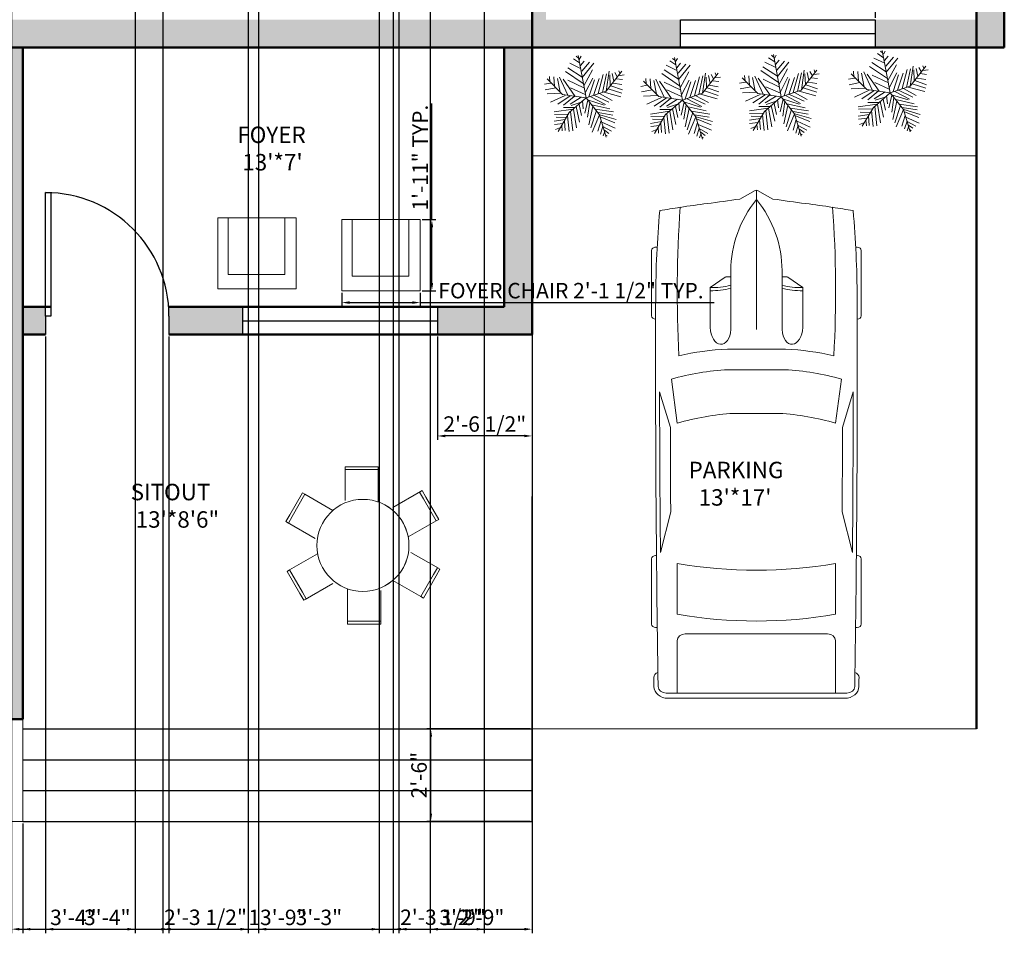
# Model space of a CAD drawing. Units: inches. Extents: x 2152 to 2718, y 1095 to 1798.
# Tile 2 of 5: x 2356 to 2675, y 1095 to 1394. Entities that reach past the tile are written whole.
import ezdxf

# ---------------------------------------------------------------- set-up
doc = ezdxf.new("R2010")
doc.units = ezdxf.units.IN
for name, color, linetype, lineweight in [('A-ANNO-DIMS', 130, 'Continuous', 18), ('A-AREA-IDEN', 130, 'Continuous', 25), ('A-FLOR-STRS', 7, 'Continuous', 25), ('A-WALL-PATT', 210, 'Continuous', 13), ('C-PRKG-VEHI', 8, 'Continuous', 13), ('DOOR', 160, 'Continuous', 25), ('FUR', 10, 'Continuous', 18), ('L-HRDS', 8, 'Continuous', 20), ('L-PLNT-BEDS', 80, 'Continuous', 18), ('TREE', 80, 'Continuous', 13), ('WALL', 7, 'Continuous', 50), ('WIND', 140, 'Continuous', 25)]:
    doc.layers.add(name, color=color, linetype=linetype, lineweight=lineweight)
doc.styles.get("Standard").update_dxf_attribs({"font": 'arial.ttf'})
doc.dimstyles.new('ISO-25', dxfattribs={"dimtxt": 5, "dimasz": 2.5, "dimexe": 1.25, "dimexo": 0.625, "dimtad": 1, "dimdec": 0, "dimlunit": 4, "dimtxsty": 'Standard', "dimcen": 2.5, "dimadec": 0, "dimazin": 0, "dimtfac": 1, "dimtdec": 0, "dimtmove": 0, "dimatfit": 3, "dimfxl": 1, "dimarcsym": 0})

# ---------------------------------------------------------------- blocks, each defined once
blk = doc.blocks.new('*U6')
for p, q in [((-10.186, 53.64), (-13.084, 55.962)), ((0, 0), (-10.5, 57)), ((-9.099, 51.782), (-6.563, 55.962)), ((-5.114, 28.097), (-24.676, 40.636)), ((-7.288, 39.707), (-21.778, 46.673)), ((-8.737, 47.138), (-17.069, 52.711)), ((-7.65, 43.423), (-2.578, 49.46)), ((-5.839, 35.992), (4.667, 48.067)), ((-5.114, 27.632), (10.463, 46.673)), ((-48.585, 21.131), (-49.309, 29.026)), ((-43.513, 28.561), (-42.427, 15.558)), ((-35.544, 28.097), (-24.314, 3.947)), ((-3.665, 19.273), (-27.574, 35.527)), ((-2.941, 16.486), (8.652, 37.85)), ((-1.129, 6.734), (9.014, 26.704)), ((16.259, 5.805), (23.142, 31.348)), ((22.055, 7.198), (27.489, 32.277)), ((27, 9), (48, 36)), ((27.127, 9.056), (31.112, 35.992)), ((31.836, 30.883), (32.561, 16.486)), ((35.096, 32.741), (37.27, 22.524)), ((38.719, 34.134), (41.979, 28.561)), ((43.791, 29.954), (51.036, 30.883)), ((44.153, 36.456), (45.239, 32.741)), ((-47.498, 19.737), (-55.83, 18.344)), ((-40.615, 13.7), (-55.105, 10.913)), ((-31.5, 4.5), (-52.5, 25.5)), ((-38.442, 26.239), (-34.819, 7.663)), ((-14.533, 2.09), (-30.834, 25.31)), ((-24.314, 23.917), (-2.941, 13.7)), ((-20.691, 13.7), (-1.129, 4.876)), ((3.942, 1.625), (11.187, 24.381)), ((10.101, 3.483), (17.708, 26.239)), ((33.285, 16.486), (48.862, 10.913)), ((36.183, 19.737), (48.137, 17.88)), ((40.53, 25.775), (48.862, 24.846)), ((-33.37, 6.269), (-52.207, 5.34)), ((-28.299, 3.483), (-47.86, -5.805)), ((-21.416, 3.018), (-38.079, -8.128)), ((0, 0), (-31.5, 4.5)), ((-15.982, 2.09), (-30.11, -9.521)), ((0, 0), (-22.5, -19.5)), ((-6.563, 1.161), (-21.416, -8.128)), ((0, 0), (27, 9)), ((0, 0), (18, -22.5)), ((6.478, 1.625), (26.04, -8.592)), ((11.187, 3.483), (30.749, -5.805)), ((18.07, 5.805), (35.096, -3.483)), ((24.229, 7.663), (46.688, 1.625)), ((29.662, 12.307), (48.137, 6.269)), ((-15.257, -12.772), (-30.11, -12.772)), ((-6.563, -5.805), (-19.967, -9.985)), ((-13.446, -11.378), (-8.737, -32.741)), ((-9.461, -8.592), (-6.201, -23.453)), ((-4.752, -3.483), (-3.665, -14.629)), ((2.493, -3.019), (-1.491, -20.202)), ((1.769, -2.555), (24.229, -9.521)), ((5.029, -6.27), (2.131, -25.775)), ((9.014, -11.378), (3.58, -35.992)), ((7.565, -9.056), (32.198, -14.629)), ((-17.431, -15.094), (-42.789, -18.809)), ((-24.314, -21.596), (-42.427, -22.06)), ((-26.849, -26.24), (-40.253, -25.775)), ((-22.5, -19.5), (-37.5, -45)), ((-25.038, -23.918), (-22.865, -45.281)), ((-20.691, -18.345), (-17.793, -44.352)), ((-17.069, -15.094), (-12.721, -40.172)), ((14.085, -16.951), (6.478, -40.172)), ((18.07, -22.524), (8.289, -45.745)), ((12.274, -15.094), (36.907, -18.809)), ((16.259, -19.738), (36.183, -22.989)), ((18, -22.5), (27, -52.5)), ((18.433, -22.524), (40.53, -29.026)), ((19.157, -25.311), (38.719, -33.206)), ((-28.299, -29.026), (-42.789, -31.348)), ((-30.834, -34.135), (-42.427, -35.528)), ((-34.457, -39.708), (-40.978, -42.494)), ((-32.646, -36.921), (-31.921, -44.352)), ((-29.023, -30.884), (-27.936, -43.887)), ((20.244, -30.419), (15.897, -44.816)), ((22.78, -37.85), (19.519, -48.532)), ((21.331, -32.741), (39.081, -40.636)), ((22.78, -38.314), (34.372, -44.816)), ((24.591, -45.745), (23.142, -50.854)), ((24.591, -43.423), (30.749, -47.603)), ((26.764, -49.925), (28.213, -50.854))]:
    blk.add_line(p, q)
blk = doc.blocks.new('*U4')
for p, q in [((21.1, 37.41), (21.1, 36.83)), ((46.55, 38.89), (22.35, 38.89)), ((47.8, 37.39), (47.8, 37.41)), ((135.45, 37.07), (135.45, 37.41)), ((136.7, 38.89), (160.9, 38.89)), ((162.15, 37.41), (162.15, 36.77)), ((87.99, 31.87), (74.76, 35.92)), ((134.31, 35.6), (119.29, 31.78)), ((186.47, -33.5), (186.47, 33.5)), ((70.03, 31.54), (86.41, 29.35)), ((138.42, 29.35), (157.25, 29.35)), ((186.47, 29.35), (167.01, 29.35)), ((188.4, -32.76), (188.4, 32.76)), ((164.52, 26.39), (164.52, -26.39)), ((32.27, 11.63), (36.13, 17.17)), ((36.13, 17.17), (50.94, 17.17)), ((32.12, 9.51), (32.12, 11.15)), ((29.77, 9.51), (51.68, 9.51)), ((58.92, -10.77), (58.92, 10.77)), ((66.55, -10.53), (66.55, 10.53)), ((82.74, 8.5), (82.74, -8.5)), ((186.47, -10.53), (186.47, 10.53)), ((3.27, 6.13), (0.1, 0.41)), ((0, 0), (51.68, 0)), ((0.1, -0.41), (3.27, -6.13)), ((29.77, -9.51), (51.68, -9.51)), ((32.12, -9.51), (32.12, -11.15)), ((32.27, -11.63), (36.13, -17.17)), ((36.13, -17.17), (50.94, -17.17)), ((86.41, -29.35), (70.03, -31.54)), ((87.99, -31.87), (74.76, -35.92)), ((134.31, -35.6), (119.29, -31.78)), ((157.25, -29.35), (138.42, -29.35)), ((167.01, -29.35), (186.47, -29.35)), ((21.1, -37.41), (21.1, -36.83)), ((46.55, -38.89), (22.35, -38.89)), ((47.8, -37.39), (47.8, -37.41)), ((135.45, -37.07), (135.45, -37.41)), ((136.7, -38.89), (160.9, -38.89)), ((162.15, -37.41), (162.15, -36.77))]:
    blk.add_line(p, q)
for centre, major_axis, ratio, start_param, end_param in [((41.19, -490.86), (0, 528.23), 0.842304, 0.00281, 0.075598), ((22.35, 37.41), (0, -1.48), 0.842304, 3.141593, 4.712389), ((64.48, -10555.62), (0, 10593.03), 0.842304, -0.013397, 0.002797), ((46.55, 37.41), (0, 1.48), 0.842304, -1.570796, 0), ((136.7, 37.41), (0, -1.48), 0.842304, 3.141593, 4.712389), ((160.9, 37.41), (0, 1.48), 0.842304, -1.570796, 0), ((180.63, 35.84), (0, 2.22), 0.842304, -0.013017, 1.249894), ((64.48, -10556.36), (0, 10595.31), 0.842304, -0.013397, -0.013017), ((183.98, 32.76), (0, -5.25), 0.842304, 1.570796, 3.128196), ((266.03, -27.52), (0, 313.31), 0.842304, 1.367076, 1.39176), ((64.48, -10555.62), (0, -10591.55), 0.842304, 3.133765, 3.140441), ((183.98, 33.5), (0, -2.96), 0.842304, 1.570796, 3.128196), ((37.47, -593.96), (0, -623.33), 0.842304, 3.096046, 3.200911), ((135.29, 5.39), (0, 81.77), 0.842304, 1.245306, 1.50788), ((149.6, 2.8), (0, -79.58), 0.842304, 4.372215, 4.640744), ((95.79, -3666.35), (0, -3698.24), 0.842304, 3.134049, 3.144098), ((17.08, 0), (0, 147.02), 0.842304, 4.511394, 4.913384), ((35.91, 0), (0, 147.02), 0.842304, 4.511394, 4.913384), ((167.01, 26.39), (0, 2.96), 0.842304, 0, 1.570796), ((259.18, -27.52), (0, -305.3), 0.842304, 4.528606, 4.561838), ((134.4, 5.39), (0, -89.78), 0.842304, 4.449482, 4.652344), ((-204.49, 52.4), (0, -250.96), 0.842304, 1.385369, 1.434372), ((13.04, 17.01), (0, 27.42), 0.842304, 4.435146, 4.718221), ((14.2, 17.01), (0, 27.42), 0.842304, 4.435146, 4.718221), ((50.79, 13.34), (6.34, -0.36), 0.603834, -1.395552, 1.581315), ((32.75, 11.15), (0, 0.74), 0.842304, 0.879714, 1.570796), ((29.77, -46.66), (0, 56.17), 0.842304, 0, 0.590319), ((0.62, 0), (0, -0.74), 0.842304, 4.131459, 5.293319), ((29.77, 46.66), (0, 56.17), 0.842304, 2.551274, 3.141593), ((-204.49, -52.4), (0, 250.96), 0.842304, -1.434372, -1.385369), ((13.04, -17.01), (0, -27.42), 0.842304, 1.564964, 1.848039), ((14.2, -17.01), (0, -27.42), 0.842304, 1.564964, 1.848039), ((134.4, -5.39), (0, -89.78), 0.842304, -1.510751, -1.307889), ((135.29, -5.39), (0, -81.77), 0.842304, -1.50788, -1.245306), ((149.6, -2.8), (0, -79.58), 0.842304, -1.499151, -1.230623), ((32.75, -11.15), (0, -0.74), 0.842304, 4.712389, 5.403472), ((259.18, 27.52), (0, 305.3), 0.842304, 1.721348, 1.754579), ((266.03, 27.52), (0, 313.31), 0.842304, 1.749832, 1.774517), ((37.47, 593.96), (0, -623.33), 0.842304, -0.059319, 0.045547), ((167.01, -26.39), (0, -2.96), 0.842304, 4.712389, 6.283185), ((95.79, 3666.35), (0, -3698.24), 0.842304, -0.002505, 0.007544), ((183.98, -32.76), (0, -5.25), 0.842304, 0.013397, 1.570796), ((41.19, 490.86), (0, -528.23), 0.842304, -0.075598, -0.00281), ((64.48, 10555.62), (0, 10593.03), 0.842304, 3.138796, 3.15499), ((64.48, 10555.62), (0, -10591.55), 0.842304, 0.001152, 0.007828), ((183.98, -33.5), (0, 2.96), 0.842304, 3.15499, 4.712389), ((22.35, -37.41), (0, 1.48), 0.842304, 1.570796, 3.141593), ((46.55, -37.41), (0, -1.48), 0.842304, 0, 1.570796), ((136.7, -37.41), (0, -1.48), 0.842304, -1.570796, 0), ((160.9, -37.41), (0, 1.48), 0.842304, 3.141593, 4.712389), ((180.63, -35.84), (0, -2.22), 0.842304, -1.249894, 0.013017), ((64.48, 10556.36), (0, 10595.31), 0.842304, 3.15461, 3.15499)]:
    blk.add_ellipse(centre, major_axis=major_axis, ratio=ratio, start_param=start_param, end_param=end_param)
at = {"extrusion": (0, 0, -1)}
blk.add_ellipse((50.79, -13.34), major_axis=(6.34, 0.36), ratio=0.603834, start_param=-1.395552, end_param=1.581315, dxfattribs=at)
blk = doc.blocks.new('*U2')
for p, q in [((0, 0), (0, -6)), ((40, 0), (40, -6))]:
    blk.add_line(p, q)
blk.add_lwpolyline([(0, 0), (0, 40), (1.75, 40), (1.75, 0)], close=True)
blk.add_arc((0, 0), 40, 0, 90)
blk = doc.blocks.new('*U11')
for p, q in [((-3.3, 20.2), (-5.8, 20.2)), ((-5.8, 20.2), (-5.8, 19.25)), ((-5.8, 9.27), (-5.8, 19.61)), ((-3.3, 19.25), (-5.8, 19.25)), ((-3.3, 20.2), (4.97, 20.2)), ((4.97, 19.25), (-3.3, 19.25)), ((4.97, 20.2), (4.97, 19.25)), ((4.97, 8.78), (4.97, 19.25))]:
    blk.add_line(p, q)
blk.add_circle((0, -5.28), 14.92)
blk = doc.blocks.new('*U12')
at = {"layer": 'FUR', "transparency": 16777216}
for p, rotation in [((1270.89, 785.87), 59.99999999999999), ((1280.04, 785.87), 300), ((1270.89, 780.59), 120), ((1280.04, 780.59), 240), ((1275.47, 777.95), 180)]:
    blk.add_blockref('*U11', p, dxfattribs=dict(at, rotation=rotation))
blk.add_blockref('*U11', (1275.47, 788.51), dxfattribs=at)
blk = doc.blocks.new('WIN-WIDE')
blk.add_line((0, 4.5), (63.07, 4.5))
blk.add_lwpolyline([(0, 9), (63.07, 9), (63.07, 0), (0, 0)], close=True)
blk = doc.blocks.new('FOYER-CHAIR')
for p, q in [((3.33, 23.07), (3.33, 4.69)), ((21.69, 23.07), (21.69, 4.69)), ((3.33, 4.69), (21.69, 4.69))]:
    blk.add_line(p, q)
blk.add_lwpolyline([(0, 0), (25.36, 0), (25.36, 23.07), (0, 23.07)], close=True)
blk = doc.blocks.new('*D30')
at = {"layer": 'A-ANNO-DIMS', "color": 0, "lineweight": -2, "transparency": 16777216}
for p, q in [((2460.42, 1305.44), (2460.42, 1301.01)), ((2485.78, 1305.44), (2485.78, 1301.01)), ((2462.92, 1302.26), (2483.28, 1302.26)), ((2485.78, 1302.26), (2581.06, 1302.26))]:
    blk.add_line(p, q, dxfattribs=at)
at = {"layer": 'A-ANNO-DIMS', "color": 0, "transparency": 16777216}
for points in [[(2462.92, 1302.68), (2462.92, 1301.84), (2460.42, 1302.26)], [(2483.28, 1302.68), (2483.28, 1301.84), (2485.78, 1302.26)]]:
    blk.add_solid(points, dxfattribs=at)
at = {"layer": 'Defpoints', "color": 0, "transparency": 16777216}
for p in [(2460.42, 1306.07), (2485.78, 1306.07), (2485.78, 1302.26)]:
    blk.add_point(p, dxfattribs=at)
at = {"layer": 'A-ANNO-DIMS', "color": 0, "transparency": 16777216, "insert": (2534.67, 1305.47), "char_height": 5, "attachment_point": 5}
blk.add_mtext('FOYER CHAIR 2\'-1 1/2" TYP.', dxfattribs=at)
blk = doc.blocks.new('*D31')
at = {"layer": 'A-ANNO-DIMS', "color": 0, "lineweight": -2, "transparency": 16777216}
for p, q in [((2489.59, 1329.13), (2489.59, 1366.77)), ((2486.41, 1329.13), (2490.84, 1329.13)), ((2489.59, 1308.57), (2489.59, 1326.63)), ((2486.41, 1306.07), (2490.84, 1306.07))]:
    blk.add_line(p, q, dxfattribs=at)
at = {"layer": 'A-ANNO-DIMS', "color": 0, "transparency": 16777216}
for points in [[(2489.17, 1326.63), (2490.01, 1326.63), (2489.59, 1329.13)], [(2489.17, 1308.57), (2490.01, 1308.57), (2489.59, 1306.07)]]:
    blk.add_solid(points, dxfattribs=at)
at = {"layer": 'Defpoints', "color": 0, "transparency": 16777216}
for p in [(2485.78, 1329.13), (2489.59, 1329.13), (2485.78, 1306.07)]:
    blk.add_point(p, dxfattribs=at)
at = {"layer": 'A-ANNO-DIMS', "color": 0, "transparency": 16777216, "insert": (2486.45, 1349.2), "char_height": 5, "attachment_point": 5, "rotation": 90}
blk.add_mtext('1\'-11" TYP.', dxfattribs=at)
blk = doc.blocks.new('*D43')
at = {"layer": 'A-ANNO-DIMS', "color": 0, "lineweight": -2, "transparency": 16777216}
for p, q in [((2491.42, 1291.24), (2491.42, 1257.82)), ((2522.06, 1291.24), (2522.06, 1257.82)), ((2519.56, 1259.07), (2493.92, 1259.07))]:
    blk.add_line(p, q, dxfattribs=at)
at = {"layer": 'A-ANNO-DIMS', "color": 0, "transparency": 16777216}
for points in [[(2493.92, 1259.48), (2493.92, 1258.65), (2491.42, 1259.07)], [(2519.56, 1259.48), (2519.56, 1258.65), (2522.06, 1259.07)]]:
    blk.add_solid(points, dxfattribs=at)
at = {"layer": 'Defpoints', "color": 0, "transparency": 16777216}
for p in [(2491.42, 1291.87), (2522.06, 1291.87), (2491.42, 1259.07)]:
    blk.add_point(p, dxfattribs=at)
at = {"layer": 'A-ANNO-DIMS', "color": 0, "transparency": 16777216, "insert": (2506.74, 1262.28), "char_height": 5, "attachment_point": 5}
blk.add_mtext('2\'-6 1/2"', dxfattribs=at)
blk = doc.blocks.new('*D44')
at = {"layer": 'A-ANNO-DIMS', "color": 0, "lineweight": -2, "transparency": 16777216}
for p, q in [((2633.28, 1394.49), (2633.28, 1788.86)), ((2635.78, 1787.61), (2663.56, 1787.61)), ((2666.06, 1394.49), (2666.06, 1788.86))]:
    blk.add_line(p, q, dxfattribs=at)
at = {"layer": 'A-ANNO-DIMS', "color": 0, "transparency": 16777216}
for points in [[(2635.78, 1788.03), (2635.78, 1787.19), (2633.28, 1787.61)], [(2663.56, 1788.03), (2663.56, 1787.19), (2666.06, 1787.61)]]:
    blk.add_solid(points, dxfattribs=at)
at = {"layer": 'Defpoints', "color": 0, "transparency": 16777216}
for p in [(2666.06, 1787.61), (2633.28, 1393.87), (2666.06, 1393.87)]:
    blk.add_point(p, dxfattribs=at)
at = {"layer": 'A-ANNO-DIMS', "color": 0, "transparency": 16777216, "insert": (2649.67, 1790.79), "char_height": 5, "attachment_point": 5}
blk.add_mtext('2\'-9"', dxfattribs=at)
blk = doc.blocks.new('*D46')
at = {"layer": 'A-ANNO-DIMS', "color": 0, "lineweight": -2, "transparency": 16777216}
for p, q in [((2364.43, 1291.24), (2364.43, 1098.09)), ((2404.43, 1291.24), (2404.43, 1098.09)), ((2366.93, 1099.34), (2401.93, 1099.34))]:
    blk.add_line(p, q, dxfattribs=at)
at = {"layer": 'A-ANNO-DIMS', "color": 0, "transparency": 16777216}
for points in [[(2366.93, 1099.75), (2366.93, 1098.92), (2364.43, 1099.34)], [(2401.93, 1099.75), (2401.93, 1098.92), (2404.43, 1099.34)]]:
    blk.add_solid(points, dxfattribs=at)
at = {"layer": 'Defpoints', "color": 0, "transparency": 16777216}
for p in [(2364.43, 1291.87), (2404.43, 1291.87), (2404.43, 1099.34)]:
    blk.add_point(p, dxfattribs=at)
at = {"layer": 'A-ANNO-DIMS', "color": 0, "transparency": 16777216, "insert": (2384.43, 1102.51), "char_height": 5, "attachment_point": 5}
blk.add_mtext('3\'-4"', dxfattribs=at)
blk = doc.blocks.new('*D52')
at = {"layer": 'A-ANNO-DIMS', "color": 0, "lineweight": -2, "transparency": 16777216}
for p, q in [((2402.42, 1648.24), (2402.42, 1098.09)), ((2430.09, 1648.24), (2430.09, 1098.09)), ((2404.92, 1099.34), (2427.59, 1099.34))]:
    blk.add_line(p, q, dxfattribs=at)
at = {"layer": 'A-ANNO-DIMS', "color": 0, "transparency": 16777216}
for points in [[(2404.92, 1099.75), (2404.92, 1098.92), (2402.42, 1099.34)], [(2427.59, 1099.75), (2427.59, 1098.92), (2430.09, 1099.34)]]:
    blk.add_solid(points, dxfattribs=at)
at = {"layer": 'Defpoints', "color": 0, "transparency": 16777216}
for p in [(2402.42, 1648.87), (2430.09, 1648.87), (2430.09, 1099.34)]:
    blk.add_point(p, dxfattribs=at)
at = {"layer": 'A-ANNO-DIMS', "color": 0, "transparency": 16777216, "insert": (2416.26, 1102.55), "char_height": 5, "attachment_point": 5}
blk.add_mtext('2\'-3 1/2"', dxfattribs=at)
blk = doc.blocks.new('*D53')
at = {"layer": 'A-ANNO-DIMS', "color": 0, "lineweight": -2, "transparency": 16777216}
for p, q in [((2353.45, 1564.24), (2353.45, 1098.09)), ((2393.45, 1564.24), (2393.45, 1098.09)), ((2355.95, 1099.34), (2390.95, 1099.34))]:
    blk.add_line(p, q, dxfattribs=at)
at = {"layer": 'A-ANNO-DIMS', "color": 0, "transparency": 16777216}
for points in [[(2355.95, 1099.75), (2355.95, 1098.92), (2353.45, 1099.34)], [(2390.95, 1099.75), (2390.95, 1098.92), (2393.45, 1099.34)]]:
    blk.add_solid(points, dxfattribs=at)
at = {"layer": 'Defpoints', "color": 0, "transparency": 16777216}
for p in [(2353.45, 1564.87), (2393.45, 1564.87), (2393.45, 1099.34)]:
    blk.add_point(p, dxfattribs=at)
at = {"layer": 'A-ANNO-DIMS', "color": 0, "transparency": 16777216, "insert": (2373.45, 1102.51), "char_height": 5, "attachment_point": 5}
blk.add_mtext('3\'-4"', dxfattribs=at)
blk = doc.blocks.new('*D54')
at = {"layer": 'A-ANNO-DIMS', "color": 0, "lineweight": -2, "transparency": 16777216}
for p, q in [((2521.43, 1164.22), (2488.01, 1164.22)), ((2489.26, 1136.72), (2489.26, 1161.72)), ((2521.43, 1134.22), (2488.01, 1134.22))]:
    blk.add_line(p, q, dxfattribs=at)
at = {"layer": 'A-ANNO-DIMS', "color": 0, "transparency": 16777216}
for points in [[(2488.84, 1161.72), (2489.68, 1161.72), (2489.26, 1164.22)], [(2488.84, 1136.72), (2489.68, 1136.72), (2489.26, 1134.22)]]:
    blk.add_solid(points, dxfattribs=at)
at = {"layer": 'Defpoints', "color": 0, "transparency": 16777216}
for p in [(2489.26, 1164.22), (2522.06, 1164.22), (2522.06, 1134.22)]:
    blk.add_point(p, dxfattribs=at)
at = {"layer": 'A-ANNO-DIMS', "color": 0, "transparency": 16777216, "insert": (2486.08, 1149.22), "char_height": 5, "attachment_point": 5, "rotation": 90}
blk.add_mtext('2\'-6"', dxfattribs=at)
blk = doc.blocks.new('*D55')
at = {"layer": 'A-ANNO-DIMS', "color": 0, "lineweight": -2, "transparency": 16777216}
for p, q in [((2357.06, 1133.59), (2357.06, 1098.09)), ((2522.06, 1133.59), (2522.06, 1098.09)), ((2359.56, 1099.34), (2519.56, 1099.34))]:
    blk.add_line(p, q, dxfattribs=at)
at = {"layer": 'A-ANNO-DIMS', "color": 0, "transparency": 16777216}
for points in [[(2359.56, 1099.75), (2359.56, 1098.92), (2357.06, 1099.34)], [(2519.56, 1099.75), (2519.56, 1098.92), (2522.06, 1099.34)]]:
    blk.add_solid(points, dxfattribs=at)
at = {"layer": 'Defpoints', "color": 0, "transparency": 16777216}
for p in [(2357.06, 1134.22), (2522.06, 1134.22), (2522.06, 1099.34)]:
    blk.add_point(p, dxfattribs=at)
at = {"layer": 'A-ANNO-DIMS', "color": 0, "transparency": 16777216, "insert": (2439.56, 1102.51), "char_height": 5, "attachment_point": 5}
blk.add_mtext('13\'-9"', dxfattribs=at)
blk = doc.blocks.new('*D56')
at = {"layer": 'A-ANNO-DIMS', "color": 0, "lineweight": -2, "transparency": 16777216}
for p, q in [((2477.06, 1564.24), (2477.06, 1098.09)), ((2522.06, 1564.24), (2522.06, 1098.09)), ((2479.56, 1099.34), (2519.56, 1099.34))]:
    blk.add_line(p, q, dxfattribs=at)
at = {"layer": 'A-ANNO-DIMS', "color": 0, "transparency": 16777216}
for points in [[(2479.56, 1099.75), (2479.56, 1098.92), (2477.06, 1099.34)], [(2519.56, 1099.75), (2519.56, 1098.92), (2522.06, 1099.34)]]:
    blk.add_solid(points, dxfattribs=at)
at = {"layer": 'Defpoints', "color": 0, "transparency": 16777216}
for p in [(2477.06, 1564.87), (2522.06, 1564.87), (2522.06, 1099.34)]:
    blk.add_point(p, dxfattribs=at)
at = {"layer": 'A-ANNO-DIMS', "color": 0, "transparency": 16777216, "insert": (2499.56, 1102.51), "char_height": 5, "attachment_point": 5}
blk.add_mtext('3\'-9"', dxfattribs=at)
blk = doc.blocks.new('*D57')
at = {"layer": 'A-ANNO-DIMS', "color": 0, "lineweight": -2, "transparency": 16777216}
for p, q in [((2489.06, 1721.19), (2489.06, 1098.09)), ((2522.06, 1710.69), (2522.06, 1098.09)), ((2491.56, 1099.34), (2519.56, 1099.34))]:
    blk.add_line(p, q, dxfattribs=at)
at = {"layer": 'A-ANNO-DIMS', "color": 0, "transparency": 16777216}
for points in [[(2491.56, 1099.75), (2491.56, 1098.92), (2489.06, 1099.34)], [(2519.56, 1099.75), (2519.56, 1098.92), (2522.06, 1099.34)]]:
    blk.add_solid(points, dxfattribs=at)
at = {"layer": 'Defpoints', "color": 0, "transparency": 16777216}
for p in [(2489.06, 1721.81), (2522.06, 1711.31), (2522.06, 1099.34)]:
    blk.add_point(p, dxfattribs=at)
at = {"layer": 'A-ANNO-DIMS', "color": 0, "transparency": 16777216, "insert": (2505.56, 1102.51), "char_height": 5, "attachment_point": 5}
blk.add_mtext('2\'-9"', dxfattribs=at)
blk = doc.blocks.new('*D59')
at = {"layer": 'A-ANNO-DIMS', "color": 0, "lineweight": -2, "transparency": 16777216}
for p, q in [((2478.92, 1660.24), (2478.92, 1098.09)), ((2506.58, 1660.24), (2506.58, 1098.09)), ((2481.42, 1099.34), (2504.08, 1099.34))]:
    blk.add_line(p, q, dxfattribs=at)
at = {"layer": 'A-ANNO-DIMS', "color": 0, "transparency": 16777216}
for points in [[(2481.42, 1099.75), (2481.42, 1098.92), (2478.92, 1099.34)], [(2504.08, 1099.75), (2504.08, 1098.92), (2506.58, 1099.34)]]:
    blk.add_solid(points, dxfattribs=at)
at = {"layer": 'Defpoints', "color": 0, "transparency": 16777216}
for p in [(2478.92, 1660.87), (2506.58, 1660.87), (2506.58, 1099.34)]:
    blk.add_point(p, dxfattribs=at)
at = {"layer": 'A-ANNO-DIMS', "color": 0, "transparency": 16777216, "insert": (2492.75, 1102.55), "char_height": 5, "attachment_point": 5}
blk.add_mtext('2\'-3 1/2"', dxfattribs=at)
blk = doc.blocks.new('*D60')
at = {"layer": 'A-ANNO-DIMS', "color": 0, "lineweight": -2, "transparency": 16777216}
for p, q in [((2433.42, 1568.74), (2433.42, 1098.09)), ((2472.56, 1568.74), (2472.56, 1098.09)), ((2435.92, 1099.34), (2470.06, 1099.34))]:
    blk.add_line(p, q, dxfattribs=at)
at = {"layer": 'A-ANNO-DIMS', "color": 0, "transparency": 16777216}
for points in [[(2435.92, 1099.75), (2435.92, 1098.92), (2433.42, 1099.34)], [(2470.06, 1099.75), (2470.06, 1098.92), (2472.56, 1099.34)]]:
    blk.add_solid(points, dxfattribs=at)
at = {"layer": 'Defpoints', "color": 0, "transparency": 16777216}
for p in [(2433.42, 1569.37), (2472.56, 1569.37), (2472.56, 1099.34)]:
    blk.add_point(p, dxfattribs=at)
at = {"layer": 'A-ANNO-DIMS', "color": 0, "transparency": 16777216, "insert": (2452.99, 1102.51), "char_height": 5, "attachment_point": 5}
blk.add_mtext('3\'-3"', dxfattribs=at)

msp = doc.modelspace()

# ---------------------------------------------------------------- hatches: boundary and pattern name
at = {"layer": 'A-WALL-PATT'}
h = msp.add_hatch(color=256, dxfattribs=at)
h.dxf.hatch_style = 1
h.paths.add_polyline_path([(2204.06, 1737.37), (2275.93, 1737.37), (2275.93, 1746.37), (2195.06, 1746.37), (2195.06, 1548.16), (2204.06, 1548.16)])
h.paths.add_polyline_path([(2567.46, 1746.37), (2519.79, 1746.37), (2519.79, 1737.37), (2549.06, 1737.37), (2567.46, 1737.37)])
h.paths.add_polyline_path([(2526.56, 1706.63), (2526.56, 1737.37), (2522.06, 1737.37), (2522.06, 1614.04), (2526.56, 1614.04), (2526.56, 1660.87)])
h.paths.add_polyline_path([(2477.06, 1737.37), (2472.56, 1737.37), (2472.56, 1653.37), (2430.09, 1653.37), (2430.09, 1648.87), (2472.56, 1648.87), (2472.56, 1569.37), (2400.56, 1569.37), (2400.56, 1573.72), (2399.94, 1573.72), (2396.06, 1573.72), (2396.06, 1569.37), (2393.45, 1569.37), (2393.45, 1564.87), (2477.06, 1564.87), (2477.06, 1648.87)])
h.paths.add_polyline_path([(2400.56, 1737.37), (2396.06, 1737.37), (2396.06, 1599.61), (2400.56, 1599.61), (2400.56, 1648.87), (2402.42, 1648.87), (2402.42, 1653.37), (2400.56, 1653.37)], flags=17)
h.paths.add_polyline_path([(2353.45, 1569.37), (2204.06, 1569.37), (2204.06, 1564.87), (2353.45, 1564.87)])
h.paths.add_polyline_path([(2280.56, 1492.87), (2221.07, 1492.87), (2221.07, 1488.37), (2280.56, 1488.37)])
h.paths.add_polyline_path([(2221.07, 1492.87), (2204.06, 1492.87), (2204.06, 1488.37), (2221.07, 1488.37)])
h.paths.add_polyline_path([(2280.56, 1536.59), (2276.9, 1536.59, -0.008622), (2276.06, 1536.6), (2276.06, 1492.87), (2280.56, 1492.87)])
h.paths.add_polyline_path([(2280.56, 1564.87), (2276.06, 1564.87), (2276.06, 1560.98), (2276.9, 1560.98), (2280.56, 1560.98)])
h.paths.add_polyline_path([(2675.06, 1746.37), (2630.54, 1746.37), (2630.54, 1737.37), (2666.06, 1737.37), (2666.06, 1384.87), (2675.06, 1384.87)])
h.paths.add_polyline_path([(2666.06, 1569.37), (2578.28, 1569.37), (2526.56, 1569.37), (2526.56, 1574.04), (2522.06, 1574.04), (2522.06, 1564.87), (2522.06, 1560.6), (2526.56, 1560.6), (2526.56, 1564.87), (2666.06, 1564.87)])
h.paths.add_polyline_path([(2526.56, 1520.6), (2522.06, 1520.6), (2522.06, 1384.87), (2570.2, 1384.87), (2570.2, 1393.87), (2526.56, 1393.87)])
h.paths.add_polyline_path([(2666.06, 1393.87), (2633.28, 1393.87), (2633.28, 1384.87), (2666.06, 1384.87)], flags=17)
h.paths.add_polyline_path([(2522.06, 1393.87), (2306.06, 1393.87), (2280.56, 1393.87), (2280.56, 1384.87), (2301.56, 1384.87), (2522.06, 1384.87)])
h.paths.add_polyline_path([(2280.56, 1393.87), (2204.06, 1393.87), (2204.06, 1384.87), (2232.43, 1384.87), (2280.56, 1384.87)])
h.paths.add_polyline_path([(2204.06, 1509.71), (2195.06, 1509.71), (2195.06, 1364.72), (2204.06, 1364.72), (2204.06, 1384.87)])
h.paths.add_polyline_path([(2204.06, 1326.27), (2195.06, 1326.27), (2195.06, 1302.62), (2201.06, 1302.62), (2204.06, 1302.62), (2204.06, 1308.37)])
h.paths.add_polyline_path([(2280.56, 1384.87), (2276.06, 1384.87), (2276.06, 1312.87), (2273.63, 1312.87), (2273.63, 1312.11), (2273.63, 1308.37), (2280.56, 1308.37)])
h.paths.add_polyline_path([(2248.67, 1312.11, -0.007577), (2248.69, 1312.87), (2204.06, 1312.87), (2204.06, 1308.37), (2248.67, 1308.37)])
h.paths.add_polyline_path([(2364.43, 1297.87), (2364.43, 1300.87), (2357.06, 1300.87), (2357.06, 1291.87), (2364.43, 1291.87)])
h.paths.add_polyline_path([(2428.34, 1300.87), (2404.32, 1300.87, -0.01877), (2404.43, 1297.87), (2404.43, 1291.87), (2428.34, 1291.87)])
h.paths.add_polyline_path([(2522.06, 1384.87), (2513.06, 1384.87), (2513.06, 1300.87), (2491.42, 1300.87), (2491.42, 1291.87), (2522.06, 1291.87)])
h.paths.add_polyline_path([(2357.06, 1384.87), (2348.06, 1384.87), (2348.06, 1176.37), (2309.1, 1176.37), (2309.1, 1167.37), (2357.06, 1167.37), (2357.06, 1173.65)])
h.paths.add_polyline_path([(2475.5, 1693.24), (2504.24, 1693.24), (2504.24, 1713.14), (2475.5, 1713.14)], flags=9)

# ---------------------------------------------------------------- linework, layer by layer
at = {"layer": 'A-FLOR-STRS'}
for p, q in [((2522.06, 1134.22), (2522.06, 1239.44)), ((2357.06, 1164.22), (2522.06, 1164.22)), ((2357.06, 1154.22), (2522.06, 1154.22)), ((2357.06, 1144.22), (2522.06, 1144.22)), ((2357.06, 1134.22), (2522.06, 1134.22))]:
    msp.add_line(p, q, dxfattribs=at)
at = {"layer": 'L-HRDS'}
for p, q in [((2522.06, 1291.87), (2522.06, 1215.37)), ((2666.06, 1164.22), (2522.06, 1164.22))]:
    msp.add_line(p, q, dxfattribs=at)
at = {"layer": 'L-PLNT-BEDS'}
for p, q in [((2522.06, 1349.78), (2666.06, 1349.78)), ((2357.06, 1134.22), (2357.06, 1173.65)), ((2195.06, 1134.22), (2357.06, 1134.22))]:
    msp.add_line(p, q, dxfattribs=at)
at = {"layer": 'WALL'}
for p, q in [((2675.06, 1746.37), (2675.06, 1384.87)), ((2666.06, 1737.37), (2666.06, 1164.22)), ((2666.06, 1564.87), (2666.06, 1384.87)), ((2522.06, 1384.87), (2522.06, 1520.6)), ((2522.06, 1384.87), (2301.56, 1384.87)), ((2357.06, 1167.37), (2357.06, 1384.87)), ((2357.06, 1384.87), (2357.06, 1300.87)), ((2513.06, 1300.87), (2513.06, 1384.87)), ((2666.06, 1384.87), (2522.06, 1384.87)), ((2522.06, 1291.87), (2522.06, 1384.87)), ((2666.06, 1384.87), (2675.06, 1384.87)), ((2357.06, 1300.87), (2366.18, 1300.87)), ((2404.32, 1300.87), (2513.06, 1300.87)), ((2357.06, 1291.87), (2364.43, 1291.87)), ((2404.43, 1291.87), (2522.06, 1291.87)), ((2195.06, 1167.37), (2357.06, 1167.37))]:
    msp.add_line(p, q, dxfattribs=at)

# ---------------------------------------------------------------- block references
at = {"layer": 'C-PRKG-VEHI', "xscale": 0.8733884986913484, "yscale": 0.8733884986913484, "zscale": 0.8733884986913484, "rotation": 270}
msp.add_blockref('*U4', (2594.75, 1338.65), dxfattribs=at)
at = {"layer": 'DOOR'}
msp.add_blockref('*U2', (2364.43, 1297.87), dxfattribs=at)
at = {"layer": 'FUR'}
for name, p in [('FOYER-CHAIR', (2420.23, 1306.68)), ('FOYER-CHAIR', (2460.42, 1306.07)), ('*U12', (1191.79, 440.39))]:
    msp.add_blockref(name, p, dxfattribs=at)
at = {"layer": 'TREE', "xscale": 0.2409617007831742, "yscale": 0.2409617007831742, "zscale": 0.2409617007831742}
for p in [(2539.55, 1368.52), (2570.76, 1367.86), (2602.77, 1368.85), (2638.06, 1370.18)]:
    msp.add_blockref('*U6', p, dxfattribs=at)
at = {"layer": 'WIND'}
for p in [(2570.2, 1384.87), (2428.34, 1291.87)]:
    msp.add_blockref('WIN-WIDE', p, dxfattribs=at)

# ---------------------------------------------------------------- texts
at = {"layer": 'A-AREA-IDEN', "char_height": 5.331, "attachment_point": 1}
for s, insert in [("FOYER\\P 13'*7'", (2426.56, 1359.26)), ("PARKING\\P  13'*17'", (2572.77, 1250.71)), ('SITOUT\\P 13\'*8\'6"', (2392.01, 1243.57))]:
    msp.add_mtext_dynamic_manual_height_columns(s, width=138.497, gutter_width=26.66, heights=[0], dxfattribs=dict(at, insert=insert))

# ---------------------------------------------------------------- dimensions: what is measured, and where the dimension line sits
at = {"layer": 'A-ANNO-DIMS'}
for base, p1, p2, picture, middle in [((2666.06, 1787.61), (2633.28, 1393.87), (2666.06, 1393.87), '*D44', (2649.67, 1790.79)), ((2522.06, 1099.34), (2489.06, 1721.81), (2522.06, 1711.31), '*D57', (2505.56, 1102.51)), ((2506.58, 1099.34), (2478.92, 1660.87), (2506.58, 1660.87), '*D59', (2492.75, 1102.55)), ((2430.09, 1099.34), (2402.42, 1648.87), (2430.09, 1648.87), '*D52', (2416.26, 1102.55)), ((2472.56, 1099.34), (2433.42, 1569.37), (2472.56, 1569.37), '*D60', (2452.99, 1102.51)), ((2393.45, 1099.34), (2353.45, 1564.87), (2393.45, 1564.87), '*D53', (2373.45, 1102.51)), ((2522.06, 1099.34), (2477.06, 1564.87), (2522.06, 1564.87), '*D56', (2499.56, 1102.51)), ((2404.43, 1099.34), (2364.43, 1291.87), (2404.43, 1291.87), '*D46', (2384.43, 1102.51)), ((2522.06, 1099.34), (2357.06, 1134.22), (2522.06, 1134.22), '*D55', (2439.56, 1102.51))]:
    dim = msp.add_linear_dim(base=base, p1=p1, p2=p2, dimstyle='ISO-25', override={"dimdec": 1, "dimlfac": 1, "dimrnd": 0, "dimzin": 1, "dimdsep": 46, "dimlunit": 4, "dimfrac": 2}, dxfattribs=at)
    dim.commit()
    dim.dimension.update_dxf_attribs({"geometry": picture, "text_midpoint": middle})
dim = msp.add_linear_dim(base=(2489.59, 1329.13), p1=(2485.78, 1306.07), p2=(2485.78, 1329.13), angle=90, text='<> TYP.', dimstyle='ISO-25', override={"dimdec": 1, "dimlfac": 1, "dimrnd": 0, "dimzin": 1, "dimdsep": 46, "dimlunit": 4, "dimfrac": 2}, dxfattribs=at)
dim.commit()
dim.dimension.update_dxf_attribs({"geometry": '*D31', "text_midpoint": (2486.45, 1349.2)})
dim = msp.add_linear_dim(base=(2485.78, 1302.26), p1=(2460.42, 1306.07), p2=(2485.78, 1306.07), text='FOYER CHAIR <> TYP.', dimstyle='ISO-25', override={"dimdec": 1, "dimlfac": 1, "dimrnd": 0, "dimzin": 1, "dimdsep": 46, "dimlunit": 4, "dimfrac": 2}, dxfattribs=at)
dim.commit()
dim.dimension.update_dxf_attribs({"geometry": '*D30', "text_midpoint": (2534.67, 1305.47)})
for base, p1, p2, angle, picture, middle in [((2491.42, 1259.07), (2522.06, 1291.87), (2491.42, 1291.87), 180, '*D43', (2506.74, 1262.28)), ((2489.26, 1164.22), (2522.06, 1134.22), (2522.06, 1164.22), 90, '*D54', (2486.08, 1149.22))]:
    dim = msp.add_linear_dim(base=base, p1=p1, p2=p2, angle=angle, dimstyle='ISO-25', override={"dimdec": 1, "dimlfac": 1, "dimrnd": 0, "dimzin": 1, "dimdsep": 46, "dimlunit": 4, "dimfrac": 2}, dxfattribs=at)
    dim.commit()
    dim.dimension.update_dxf_attribs({"geometry": picture, "text_midpoint": middle})

doc.saveas('drawing.dxf')
